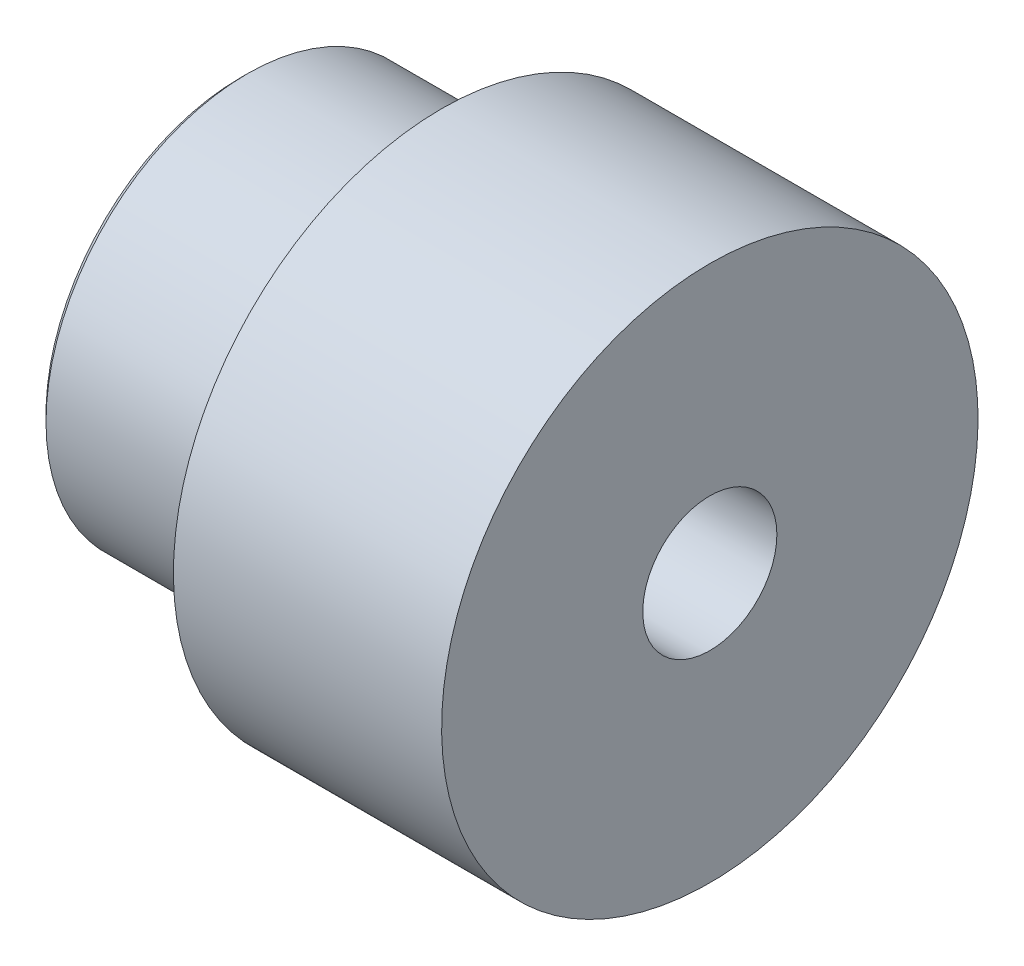
ISO-10303-21;
HEADER;
FILE_DESCRIPTION(('STEP AP214'),'2;1');
FILE_NAME('part.step','',(''),(''),'','','');
FILE_SCHEMA(('AUTOMOTIVE_DESIGN { 1 0 10303 214 1 1 1 1 }'));
ENDSEC;
DATA;
#1=APPLICATION_CONTEXT('core data for automotive mechanical design processes');
#2=APPLICATION_PROTOCOL_DEFINITION('international standard','automotive_design',2000,#1);
#3=PRODUCT_CONTEXT('',#1,'mechanical');
#4=PRODUCT('Part','Part','',(#3));
#5=PRODUCT_RELATED_PRODUCT_CATEGORY('part','',(#4));
#6=PRODUCT_DEFINITION_FORMATION('','',#4);
#7=PRODUCT_DEFINITION_CONTEXT('part definition',#1,'design');
#8=PRODUCT_DEFINITION('design','',#6,#7);
#9=PRODUCT_DEFINITION_SHAPE('','',#8);
#10=(LENGTH_UNIT() NAMED_UNIT(*) SI_UNIT(.MILLI.,.METRE.));
#11=(NAMED_UNIT(*) PLANE_ANGLE_UNIT() SI_UNIT($,.RADIAN.));
#12=(NAMED_UNIT(*) SI_UNIT($,.STERADIAN.) SOLID_ANGLE_UNIT());
#13=UNCERTAINTY_MEASURE_WITH_UNIT(LENGTH_MEASURE(1.E-05),#10,'distance_accuracy_value','');
#14=(GEOMETRIC_REPRESENTATION_CONTEXT(3) GLOBAL_UNCERTAINTY_ASSIGNED_CONTEXT((#13)) GLOBAL_UNIT_ASSIGNED_CONTEXT((#10,
#11,#12)) REPRESENTATION_CONTEXT('',''));
#15=CARTESIAN_POINT('',(0.,0.,0.));
#16=DIRECTION('',(0.,0.,1.));
#17=DIRECTION('',(1.,0.,0.));
#18=AXIS2_PLACEMENT_3D('',#15,#16,#17);
#19=CARTESIAN_POINT('',(0.,0.,0.));
#20=DIRECTION('',(1.,0.,0.));
#21=DIRECTION('',(0.,1.,0.));
#22=AXIS2_PLACEMENT_3D('',#19,#20,#21);
#23=PLANE('',#22);
#24=CARTESIAN_POINT('',(0.,0.,0.));
#25=DIRECTION('',(1.,0.,0.));
#26=DIRECTION('',(0.,0.,-1.));
#27=AXIS2_PLACEMENT_3D('',#24,#25,#26);
#28=CIRCLE('',#27,6.35);
#29=CARTESIAN_POINT('',(0.,0.,-6.35));
#30=VERTEX_POINT('',#29);
#31=EDGE_CURVE('E69',#30,#30,#28,.T.);
#32=ORIENTED_EDGE('',*,*,#31,.F.);
#33=EDGE_LOOP('',(#32));
#34=FACE_BOUND('',#33,.T.);
#35=CARTESIAN_POINT('',(0.,0.,0.));
#36=DIRECTION('',(1.,0.,0.));
#37=DIRECTION('',(0.,1.,0.));
#38=AXIS2_PLACEMENT_3D('',#35,#36,#37);
#39=CIRCLE('',#38,25.4);
#40=CARTESIAN_POINT('',(0.,25.4,0.));
#41=VERTEX_POINT('',#40);
#42=EDGE_CURVE('E93',#41,#41,#39,.T.);
#43=ORIENTED_EDGE('',*,*,#42,.T.);
#44=EDGE_LOOP('',(#43));
#45=FACE_BOUND('',#44,.T.);
#46=ADVANCED_FACE('F41',(#34,#45),#23,.T.);
#47=CARTESIAN_POINT('',(-0.941021967526265,0.,0.));
#48=DIRECTION('',(1.,0.,0.));
#49=DIRECTION('',(0.,1.,0.));
#50=AXIS2_PLACEMENT_3D('',#47,#48,#49);
#51=CYLINDRICAL_SURFACE('',#50,25.4);
#52=CARTESIAN_POINT('',(-25.4,0.,0.));
#53=DIRECTION('',(1.,0.,0.));
#54=DIRECTION('',(0.,1.,0.));
#55=AXIS2_PLACEMENT_3D('',#52,#53,#54);
#56=CIRCLE('',#55,25.4);
#57=CARTESIAN_POINT('',(-25.4,25.4,0.));
#58=VERTEX_POINT('',#57);
#59=EDGE_CURVE('E86',#58,#58,#56,.T.);
#60=ORIENTED_EDGE('',*,*,#59,.T.);
#61=EDGE_LOOP('',(#60));
#62=FACE_BOUND('',#61,.T.);
#63=ORIENTED_EDGE('',*,*,#42,.F.);
#64=EDGE_LOOP('',(#63));
#65=FACE_BOUND('',#64,.T.);
#66=ADVANCED_FACE('F112',(#62,#65),#51,.T.);
#67=CARTESIAN_POINT('',(-25.4,25.4,0.));
#68=DIRECTION('',(-1.,0.,0.));
#69=DIRECTION('',(0.,-1.,0.));
#70=AXIS2_PLACEMENT_3D('',#67,#68,#69);
#71=PLANE('',#70);
#72=CARTESIAN_POINT('',(-25.4,0.,0.));
#73=DIRECTION('',(1.,0.,0.));
#74=DIRECTION('',(0.,1.,0.));
#75=AXIS2_PLACEMENT_3D('',#72,#73,#74);
#76=CIRCLE('',#75,19.05);
#77=CARTESIAN_POINT('',(-25.4,19.05,0.));
#78=VERTEX_POINT('',#77);
#79=EDGE_CURVE('E82',#78,#78,#76,.T.);
#80=ORIENTED_EDGE('',*,*,#79,.T.);
#81=EDGE_LOOP('',(#80));
#82=FACE_BOUND('',#81,.T.);
#83=ORIENTED_EDGE('',*,*,#59,.F.);
#84=EDGE_LOOP('',(#83));
#85=FACE_BOUND('',#84,.T.);
#86=ADVANCED_FACE('F117',(#82,#85),#71,.T.);
#87=CARTESIAN_POINT('',(-0.941021967526265,0.,0.));
#88=DIRECTION('',(1.,0.,0.));
#89=DIRECTION('',(0.,1.,0.));
#90=AXIS2_PLACEMENT_3D('',#87,#88,#89);
#91=CYLINDRICAL_SURFACE('',#90,19.05);
#92=CARTESIAN_POINT('',(-43.815,0.,0.));
#93=DIRECTION('',(-1.,0.,0.));
#94=DIRECTION('',(0.,-1.,0.));
#95=AXIS2_PLACEMENT_3D('',#92,#93,#94);
#96=CIRCLE('',#95,19.05);
#97=CARTESIAN_POINT('',(-43.815,-19.05,0.));
#98=VERTEX_POINT('',#97);
#99=EDGE_CURVE('E49',#98,#98,#96,.F.);
#100=ORIENTED_EDGE('',*,*,#99,.T.);
#101=EDGE_LOOP('',(#100));
#102=FACE_BOUND('',#101,.T.);
#103=ORIENTED_EDGE('',*,*,#79,.F.);
#104=EDGE_LOOP('',(#103));
#105=FACE_BOUND('',#104,.T.);
#106=ADVANCED_FACE('F96',(#102,#105),#91,.T.);
#107=CARTESIAN_POINT('',(-44.45,0.,0.));
#108=DIRECTION('',(-1.,0.,0.));
#109=DIRECTION('',(0.,-1.,0.));
#110=AXIS2_PLACEMENT_3D('',#107,#108,#109);
#111=PLANE('',#110);
#112=CARTESIAN_POINT('',(-44.45,0.,0.));
#113=DIRECTION('',(-1.,0.,0.));
#114=DIRECTION('',(0.,-1.,0.));
#115=AXIS2_PLACEMENT_3D('',#112,#113,#114);
#116=CIRCLE('',#115,18.415);
#117=CARTESIAN_POINT('',(-44.45,-18.415,0.));
#118=VERTEX_POINT('',#117);
#119=EDGE_CURVE('E11',#118,#118,#116,.T.);
#120=ORIENTED_EDGE('',*,*,#119,.T.);
#121=EDGE_LOOP('',(#120));
#122=FACE_BOUND('',#121,.T.);
#123=CARTESIAN_POINT('',(-44.45,0.,0.));
#124=DIRECTION('',(-1.,0.,0.));
#125=DIRECTION('',(0.,0.,1.));
#126=AXIS2_PLACEMENT_3D('',#123,#124,#125);
#127=CIRCLE('',#126,3.81);
#128=CARTESIAN_POINT('',(-44.45,0.,3.81));
#129=VERTEX_POINT('',#128);
#130=EDGE_CURVE('E63',#129,#129,#127,.T.);
#131=ORIENTED_EDGE('',*,*,#130,.F.);
#132=EDGE_LOOP('',(#131));
#133=FACE_BOUND('',#132,.T.);
#134=ADVANCED_FACE('F130',(#122,#133),#111,.T.);
#135=CARTESIAN_POINT('',(-25.4,0.,0.));
#136=DIRECTION('',(-1.,0.,0.));
#137=DIRECTION('',(0.,0.,1.));
#138=AXIS2_PLACEMENT_3D('',#135,#136,#137);
#139=CONICAL_SURFACE('',#138,2.5527,1.02974425867665);
#140=CARTESIAN_POINT('',(-23.8661830978083,0.,0.));
#141=VERTEX_POINT('',#140);
#142=VERTEX_LOOP('',#141);
#143=FACE_BOUND('',#142,.T.);
#144=CARTESIAN_POINT('',(-25.4,0.,0.));
#145=DIRECTION('',(-1.,0.,0.));
#146=DIRECTION('',(0.,0.,1.));
#147=AXIS2_PLACEMENT_3D('',#144,#145,#146);
#148=CIRCLE('',#147,2.5527);
#149=CARTESIAN_POINT('',(-25.4,0.,2.5527));
#150=VERTEX_POINT('',#149);
#151=EDGE_CURVE('E81',#150,#150,#148,.T.);
#152=ORIENTED_EDGE('',*,*,#151,.T.);
#153=EDGE_LOOP('',(#152));
#154=FACE_BOUND('',#153,.T.);
#155=ADVANCED_FACE('F129',(#143,#154),#139,.F.);
#156=CARTESIAN_POINT('',(-44.45,0.,0.));
#157=DIRECTION('',(-1.,0.,0.));
#158=DIRECTION('',(0.,0.,1.));
#159=AXIS2_PLACEMENT_3D('',#156,#157,#158);
#160=CYLINDRICAL_SURFACE('',#159,2.55269999999999);
#161=ORIENTED_EDGE('',*,*,#151,.F.);
#162=EDGE_LOOP('',(#161));
#163=FACE_BOUND('',#162,.T.);
#164=CARTESIAN_POINT('',(-31.75,0.,0.));
#165=DIRECTION('',(-1.,0.,0.));
#166=DIRECTION('',(0.,0.,1.));
#167=AXIS2_PLACEMENT_3D('',#164,#165,#166);
#168=CIRCLE('',#167,2.55269999999999);
#169=CARTESIAN_POINT('',(-31.75,0.,2.55269999999999));
#170=VERTEX_POINT('',#169);
#171=EDGE_CURVE('E76',#170,#170,#168,.T.);
#172=ORIENTED_EDGE('',*,*,#171,.T.);
#173=EDGE_LOOP('',(#172));
#174=FACE_BOUND('',#173,.T.);
#175=ADVANCED_FACE('F135',(#163,#174),#160,.F.);
#176=CARTESIAN_POINT('',(-31.75,2.55269999999999,0.));
#177=DIRECTION('',(1.,0.,0.));
#178=DIRECTION('',(0.,0.,-1.));
#179=AXIS2_PLACEMENT_3D('',#176,#177,#178);
#180=PLANE('',#179);
#181=ORIENTED_EDGE('',*,*,#171,.F.);
#182=EDGE_LOOP('',(#181));
#183=FACE_BOUND('',#182,.T.);
#184=CARTESIAN_POINT('',(-31.75,0.,0.));
#185=DIRECTION('',(-1.,0.,0.));
#186=DIRECTION('',(0.,0.,1.));
#187=AXIS2_PLACEMENT_3D('',#184,#185,#186);
#188=CIRCLE('',#187,3.17499999999999);
#189=CARTESIAN_POINT('',(-31.75,0.,3.17499999999999));
#190=VERTEX_POINT('',#189);
#191=EDGE_CURVE('E77',#190,#190,#188,.T.);
#192=ORIENTED_EDGE('',*,*,#191,.T.);
#193=EDGE_LOOP('',(#192));
#194=FACE_BOUND('',#193,.T.);
#195=ADVANCED_FACE('F139',(#183,#194),#180,.F.);
#196=CARTESIAN_POINT('',(-44.45,0.,0.));
#197=DIRECTION('',(-1.,0.,0.));
#198=DIRECTION('',(0.,0.,1.));
#199=AXIS2_PLACEMENT_3D('',#196,#197,#198);
#200=CYLINDRICAL_SURFACE('',#199,3.17499999999999);
#201=ORIENTED_EDGE('',*,*,#191,.F.);
#202=EDGE_LOOP('',(#201));
#203=FACE_BOUND('',#202,.T.);
#204=CARTESIAN_POINT('',(-43.7195160614147,0.,0.));
#205=DIRECTION('',(-1.,0.,0.));
#206=DIRECTION('',(0.,0.,1.));
#207=AXIS2_PLACEMENT_3D('',#204,#205,#206);
#208=CIRCLE('',#207,3.175);
#209=CARTESIAN_POINT('',(-43.7195160614147,0.,3.175));
#210=VERTEX_POINT('',#209);
#211=EDGE_CURVE('E68',#210,#210,#208,.T.);
#212=ORIENTED_EDGE('',*,*,#211,.T.);
#213=EDGE_LOOP('',(#212));
#214=FACE_BOUND('',#213,.T.);
#215=ADVANCED_FACE('F110',(#203,#214),#200,.F.);
#216=CARTESIAN_POINT('',(-44.45,0.,0.));
#217=DIRECTION('',(-1.,0.,0.));
#218=DIRECTION('',(0.,0.,1.));
#219=AXIS2_PLACEMENT_3D('',#216,#217,#218);
#220=CONICAL_SURFACE('',#219,3.81,0.715584993317678);
#221=ORIENTED_EDGE('',*,*,#211,.F.);
#222=EDGE_LOOP('',(#221));
#223=FACE_BOUND('',#222,.T.);
#224=ORIENTED_EDGE('',*,*,#130,.T.);
#225=EDGE_LOOP('',(#224));
#226=FACE_BOUND('',#225,.T.);
#227=ADVANCED_FACE('F99',(#223,#226),#220,.F.);
#228=CARTESIAN_POINT('',(-43.815,0.,0.));
#229=DIRECTION('',(1.,0.,0.));
#230=DIRECTION('',(0.,1.,0.));
#231=AXIS2_PLACEMENT_3D('',#228,#229,#230);
#232=CONICAL_SURFACE('',#231,19.05,0.785398163397443);
#233=ORIENTED_EDGE('',*,*,#119,.F.);
#234=EDGE_LOOP('',(#233));
#235=FACE_BOUND('',#234,.T.);
#236=ORIENTED_EDGE('',*,*,#99,.F.);
#237=EDGE_LOOP('',(#236));
#238=FACE_BOUND('',#237,.T.);
#239=ADVANCED_FACE('F42',(#235,#238),#232,.T.);
#240=CARTESIAN_POINT('',(-19.05,0.,0.));
#241=DIRECTION('',(1.,0.,0.));
#242=DIRECTION('',(0.,0.,-1.));
#243=AXIS2_PLACEMENT_3D('',#240,#241,#242);
#244=CONICAL_SURFACE('',#243,6.34999999999999,1.02974425867665);
#245=CARTESIAN_POINT('',(-22.865464930825,0.,0.));
#246=VERTEX_POINT('',#245);
#247=VERTEX_LOOP('',#246);
#248=FACE_BOUND('',#247,.T.);
#249=CARTESIAN_POINT('',(-19.05,0.,0.));
#250=DIRECTION('',(1.,0.,0.));
#251=DIRECTION('',(0.,0.,-1.));
#252=AXIS2_PLACEMENT_3D('',#249,#250,#251);
#253=CIRCLE('',#252,6.34999999999999);
#254=CARTESIAN_POINT('',(-19.05,0.,-6.34999999999999));
#255=VERTEX_POINT('',#254);
#256=EDGE_CURVE('E65',#255,#255,#253,.T.);
#257=ORIENTED_EDGE('',*,*,#256,.T.);
#258=EDGE_LOOP('',(#257));
#259=FACE_BOUND('',#258,.T.);
#260=ADVANCED_FACE('F57',(#248,#259),#244,.F.);
#261=CARTESIAN_POINT('',(0.,0.,0.));
#262=DIRECTION('',(1.,0.,0.));
#263=DIRECTION('',(0.,0.,-1.));
#264=AXIS2_PLACEMENT_3D('',#261,#262,#263);
#265=CYLINDRICAL_SURFACE('',#264,6.35);
#266=ORIENTED_EDGE('',*,*,#256,.F.);
#267=EDGE_LOOP('',(#266));
#268=FACE_BOUND('',#267,.T.);
#269=ORIENTED_EDGE('',*,*,#31,.T.);
#270=EDGE_LOOP('',(#269));
#271=FACE_BOUND('',#270,.T.);
#272=ADVANCED_FACE('F56',(#268,#271),#265,.F.);
#273=CLOSED_SHELL('',(#46,#66,#86,#106,#134,#155,#175,#195,#215,#227,#239,#260,#272));
#274=MANIFOLD_SOLID_BREP('B2',#273);
#275=ADVANCED_BREP_SHAPE_REPRESENTATION('',(#18,#274),#14);
#276=SHAPE_DEFINITION_REPRESENTATION(#9,#275);
ENDSEC;
END-ISO-10303-21;
